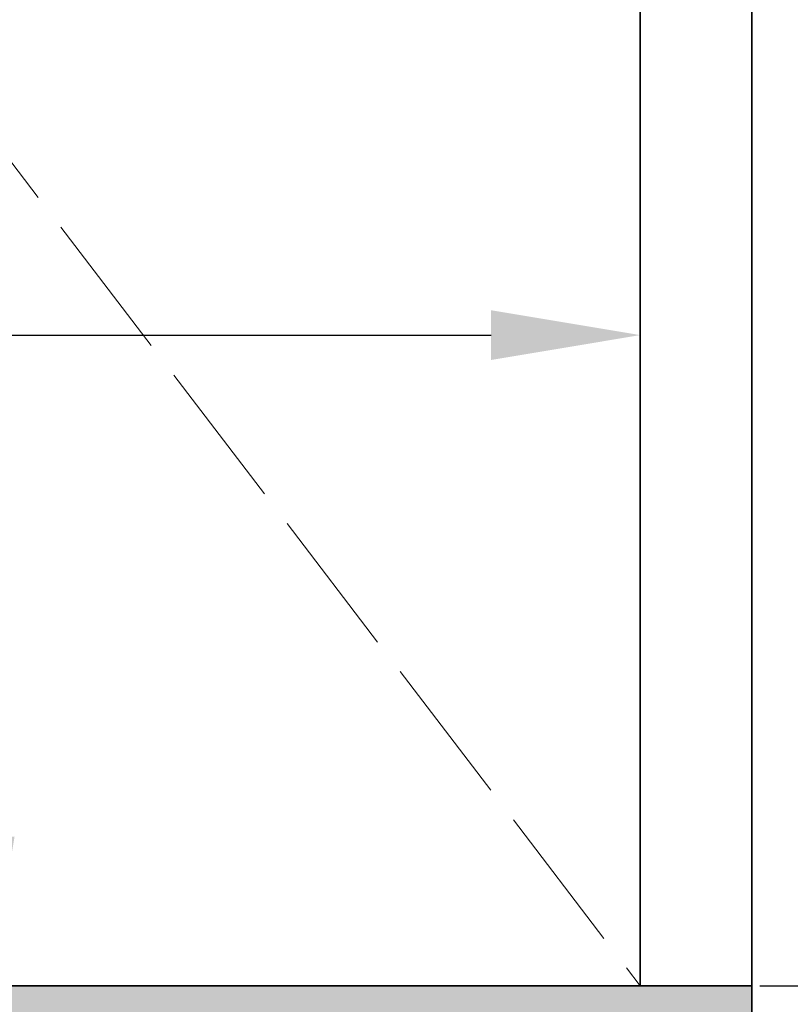
# Model space of a CAD drawing. Units: inches. Extents: x 2083 to 3317, y 1141 to 2115.
# Tile 250 of 256: x 3068 to 3130, y 1485 to 1564. Entities that reach past the tile are written whole.
import ezdxf

# ---------------------------------------------------------------- set-up
doc = ezdxf.new("R2010")
doc.units = ezdxf.units.IN
doc.linetypes.add('ACAD_ISO02W100', pattern=[15, 12, -3])
for name, color, linetype, lineweight in [('A-ANNO-DIMS', 2, 'Continuous', 18), ('A-FLOR-OPEN', 8, 'ACAD_ISO02W100', 13), ('A-WALL', 7, 'Continuous', 35)]:
    doc.layers.add(name, color=color, linetype=linetype, lineweight=lineweight)
doc.layers.add('A-WALL-PATT', color=251, linetype='Continuous', lineweight=13, true_color=0x636466)
doc.styles.get("Standard").update_dxf_attribs({"font": 'arial.ttf'})
doc.dimstyles.new('ISO-25', dxfattribs={"dimtxt": 12, "dimasz": 12, "dimexe": 1.25, "dimexo": 0.625, "dimtad": 1, "dimlunit": 3, "dimtxsty": 'Standard', "dimcen": 2.5, "dimadec": 0, "dimazin": 0, "dimtfac": 1, "dimtmove": 0, "dimatfit": 3, "dimfxl": 1, "dimarcsym": 0})

# ---------------------------------------------------------------- blocks, each defined once
blk = doc.blocks.new('*D8')
at = {"layer": 'A-ANNO-DIMS', "color": 0, "lineweight": -2, "transparency": 16777216}
for p, q in [((3127.585, 1702.761), (3191.318, 1702.761)), ((3190.068, 1690.761), (3190.068, 1498.761)), ((3127.585, 1486.761), (3191.318, 1486.761))]:
    blk.add_line(p, q, dxfattribs=at)
at = {"layer": 'A-ANNO-DIMS', "color": 0, "transparency": 16777216}
for points in [[(3188.068, 1690.761), (3192.068, 1690.761), (3190.068, 1702.761)], [(3188.068, 1498.761), (3192.068, 1498.761), (3190.068, 1486.761)]]:
    blk.add_solid(points, dxfattribs=at)
at = {"layer": 'Defpoints', "color": 0, "transparency": 16777216}
for p in [(3126.96, 1702.761), (3126.96, 1486.761), (3190.068, 1486.761)]:
    blk.add_point(p, dxfattribs=at)
at = {"layer": 'A-ANNO-DIMS', "color": 0, "transparency": 16777216, "insert": (3183.316, 1594.761), "char_height": 12, "attachment_point": 5, "rotation": 90}
blk.add_mtext("18'", dxfattribs=at)
blk = doc.blocks.new('*D9')
at = {"layer": 'A-ANNO-DIMS', "color": 0, "lineweight": -2, "transparency": 16777216}
for p, q in [((3127.585, 1486.761), (3190.403, 1486.761)), ((3189.153, 1474.761), (3189.153, 1275.261)), ((3127.585, 1263.261), (3190.403, 1263.261))]:
    blk.add_line(p, q, dxfattribs=at)
at = {"layer": 'A-ANNO-DIMS', "color": 0, "transparency": 16777216}
for points in [[(3187.153, 1474.761), (3191.153, 1474.761), (3189.153, 1486.761)], [(3187.153, 1275.261), (3191.153, 1275.261), (3189.153, 1263.261)]]:
    blk.add_solid(points, dxfattribs=at)
at = {"layer": 'Defpoints', "color": 0, "transparency": 16777216}
for p in [(3126.96, 1486.761), (3126.96, 1263.261), (3189.153, 1263.261)]:
    blk.add_point(p, dxfattribs=at)
at = {"layer": 'A-ANNO-DIMS', "color": 0, "transparency": 16777216, "insert": (3182.401, 1375.011), "char_height": 12, "attachment_point": 5, "rotation": 90}
blk.add_mtext('18\'-7.5"', dxfattribs=at)
blk = doc.blocks.new('*D35')
at = {"layer": 'A-ANNO-DIMS', "color": 0, "lineweight": -2, "transparency": 16777216}
for p, q in [((3127.585, 2020.761), (3180.56, 2020.761)), ((3179.31, 1275.261), (3179.31, 2008.761)), ((3127.585, 1263.261), (3180.56, 1263.261))]:
    blk.add_line(p, q, dxfattribs=at)
at = {"layer": 'A-ANNO-DIMS', "color": 0, "transparency": 16777216}
for points in [[(3177.31, 2008.761), (3181.31, 2008.761), (3179.31, 2020.761)], [(3177.31, 1275.261), (3181.31, 1275.261), (3179.31, 1263.261)]]:
    blk.add_solid(points, dxfattribs=at)
at = {"layer": 'Defpoints', "color": 0, "transparency": 16777216}
for p in [(3126.96, 2020.761), (3179.31, 2020.761), (3126.96, 1263.261)]:
    blk.add_point(p, dxfattribs=at)
at = {"layer": 'A-ANNO-DIMS', "color": 0, "transparency": 16777216, "insert": (3172.476, 1642.011), "char_height": 12, "attachment_point": 5, "rotation": 90}
blk.add_mtext('63\'-1 1/2"', dxfattribs=at)
blk = doc.blocks.new('*D46')
at = {"layer": 'A-ANNO-DIMS', "color": 0, "lineweight": -2, "transparency": 16777216}
for p, q in [((2952.96, 1487.386), (2952.96, 1540.361)), ((3117.96, 1487.386), (3117.96, 1540.361)), ((2964.96, 1539.111), (3105.96, 1539.111))]:
    blk.add_line(p, q, dxfattribs=at)
at = {"layer": 'A-ANNO-DIMS', "color": 0, "transparency": 16777216}
for points in [[(2964.96, 1541.111), (2964.96, 1537.111), (2952.96, 1539.111)], [(3105.96, 1541.111), (3105.96, 1537.111), (3117.96, 1539.111)]]:
    blk.add_solid(points, dxfattribs=at)
at = {"layer": 'Defpoints', "color": 0, "transparency": 16777216}
for p in [(3117.96, 1539.111), (2952.96, 1486.761), (3117.96, 1486.761)]:
    blk.add_point(p, dxfattribs=at)
at = {"layer": 'A-ANNO-DIMS', "color": 0, "transparency": 16777216, "insert": (3035.46, 1545.867), "char_height": 12, "attachment_point": 5}
blk.add_mtext('13\'-9"', dxfattribs=at)
blk = doc.blocks.new('*D65')
at = {"layer": 'A-ANNO-DIMS', "color": 0, "lineweight": -2, "transparency": 16777216}
for p, q in [((3117.335, 1702.761), (3064.36, 1702.761)), ((3065.61, 1498.761), (3065.61, 1690.761)), ((3117.335, 1486.761), (3064.36, 1486.761))]:
    blk.add_line(p, q, dxfattribs=at)
at = {"layer": 'A-ANNO-DIMS', "color": 0, "transparency": 16777216}
for points in [[(3063.61, 1690.761), (3067.61, 1690.761), (3065.61, 1702.761)], [(3063.61, 1498.761), (3067.61, 1498.761), (3065.61, 1486.761)]]:
    blk.add_solid(points, dxfattribs=at)
at = {"layer": 'Defpoints', "color": 0, "transparency": 16777216}
for p in [(3065.61, 1702.761), (3117.96, 1702.761), (3117.96, 1486.761)]:
    blk.add_point(p, dxfattribs=at)
at = {"layer": 'A-ANNO-DIMS', "color": 0, "transparency": 16777216, "insert": (3058.858, 1594.761), "char_height": 12, "attachment_point": 5, "rotation": 90}
blk.add_mtext('18\'-0"', dxfattribs=at)

msp = doc.modelspace()

# ---------------------------------------------------------------- hatches: boundary and pattern name
at = {"layer": 'A-WALL-PATT'}
h = msp.add_hatch(color=256, dxfattribs=at)
h.dxf.hatch_style = 1
h.paths.add_polyline_path([(3126.96, 2020.761), (2748.96, 2020.761), (2604.96, 2020.761), (2226.96, 2020.761), (2226.96, 1702.761), (2466.96, 1702.761), (2466.96, 1582.761), (2418.96, 1582.761), (2418.96, 1477.761), (2226.96, 1477.761), (2226.96, 1263.261), (2544.96, 1263.261), (2544.96, 1411.761), (2604.96, 1411.761), (2685.96, 1411.761), (2685.96, 1420.761), (2604.96, 1420.761), (2604.96, 1573.761), (2604.96, 1702.761), (2604.96, 2011.761), (2748.96, 2011.761), (2748.96, 1702.761), (2862.96, 1702.761), (2862.96, 1621.761), (2871.96, 1621.761), (2871.96, 1702.761), (2883.96, 1702.761), (2883.96, 1706.939, -0.026459), (2883.96, 1711.761), (2757.96, 1711.761), (2757.96, 1807.761), (2787.96, 1807.761), (2787.96, 1812.261), (2757.96, 1812.261), (2757.96, 2011.761), (2877.96, 2011.761), (2877.96, 1812.261), (2847.96, 1812.261), (2847.96, 1807.761), (2889.836, 1807.761), (2889.836, 1812.261), (2882.46, 1812.261), (2882.46, 2011.761), (3117.96, 2011.761), (3117.96, 1812.261), (2937.836, 1812.261), (2937.836, 1807.761), (2995.71, 1807.761), (2995.71, 1796.118), (3000.21, 1796.118), (3000.21, 1807.761), (3117.96, 1807.761), (3117.96, 1711.761), (3000.21, 1711.761), (3000.21, 1760.118), (2998.573, 1760.118, -0.020711), (2995.71, 1760.118), (2995.71, 1711.761), (2931.96, 1711.761), (2931.96, 1702.761), (3126.96, 1702.761)])
h.paths.add_polyline_path([(2471.46, 2011.761), (2471.46, 1810.011), (2462.717, 1810.011), (2462.717, 1805.511), (2505.96, 1805.511), (2505.96, 1810.011), (2475.96, 1810.011), (2475.96, 2011.761), (2595.96, 2011.761), (2595.96, 1810.011), (2565.96, 1810.011), (2565.96, 1805.511), (2595.96, 1805.511), (2595.96, 1711.761), (2235.96, 1711.761), (2235.96, 1805.511), (2353.71, 1805.511), (2353.71, 1796.054), (2358.21, 1796.054), (2358.21, 1805.511), (2414.717, 1805.511), (2414.717, 1810.011), (2235.96, 1810.011), (2235.96, 2011.761)], flags=16)
h.paths.add_polyline_path([(2270.205, 1994.61), (2270.205, 1970.61), (2246.205, 1970.61), (2246.205, 1994.61)], flags=0)
edge = h.paths.add_edge_path(flags=0)
edge.add_ellipse((2332.027, 1899.798), major_axis=(-3.043, 3.043), ratio=0.168252, start_angle=-161.33217, end_angle=-156.30711, ccw=False)
edge.add_ellipse((2333.082, 1898.744), major_axis=(-1.055, 1.055), ratio=0.453532, start_angle=-123.37102, end_angle=-94.15911)
edge = h.paths.add_edge_path(flags=0)
edge.add_ellipse((2332.027, 1968.876), major_axis=(3.043, 3.043), ratio=0.168252, start_angle=18.66783, end_angle=23.69289)
edge.add_spline(control_points=[(2332.926, 1970.691), (2332.227, 1970.336), (2330.894, 1969.659), (2328.413, 1970.932), (2327.204, 1967.749), (2324.71, 1969.956), (2322.533, 1967.012), (2320.013, 1971.296), (2317.68, 1968.158), (2316.041, 1967.102), (2315.427, 1966.81)], knot_values=[0, 0, 0, 0, 2.267059, 4.324559, 6.685584, 8.878641, 11.121502, 14.300359, 17.755284, 19.732645, 19.732645, 19.732645, 19.732645], degree=3, periodic=0)
edge.add_ellipse((2332.027, 1968.876), major_axis=(3.043, 3.043), ratio=0.168252, start_angle=18.66783, end_angle=23.69289, ccw=False)
edge.add_ellipse((2333.082, 1969.931), major_axis=(1.055, 1.055), ratio=0.453532, start_angle=56.62898, end_angle=85.84089, ccw=False)
edge = h.paths.add_edge_path(flags=0)
edge.add_spline(control_points=[(2296.428, 1967.988), (2293.628, 1965.336), (2287.704, 1959.727), (2299.744, 1949.996), (2294.533, 1935.669), (2290.573, 1920.604), (2293.394, 1909.974), (2296.185, 1904.967)], knot_values=[0.099185, 0.099185, 0.099185, 0.099185, 0.345301, 0.619822, 0.982653, 1.386093, 1.810555, 1.810555, 1.810555, 1.810555], degree=3, periodic=0)
edge.add_spline(control_points=[(2296.185, 1904.967), (2297.384, 1902.619), (2298.001, 1901.949), (2298.553, 1901.468)], knot_values=[0.006246, 0.006246, 0.006246, 0.006246, 0.055476, 0.055476, 0.055476, 0.055476], degree=3, periodic=0)
edge.add_spline(control_points=[(2298.553, 1901.468), (2297.259, 1900.923), (2295.225, 1900.232), (2293.06, 1900.614), (2292.101, 1900.788), (2292.09, 1900.791)], knot_values=[0.312835, 0.312835, 0.312835, 0.312835, 0.40178, 0.474987, 0.475903, 0.475903, 0.475903, 0.475903], degree=3, periodic=0)
edge.add_arc((2292.794, 1904.664), 3.937, 215.4209, 259.69818, ccw=False)
edge.add_spline(control_points=[(2289.585, 1902.382), (2289.477, 1902.535), (2289.368, 1902.688), (2289.261, 1902.841)], knot_values=[0.102872, 0.102872, 0.102872, 0.102872, 0.116896, 0.116896, 0.116896, 0.116896], degree=3, periodic=0)
edge.add_spline(control_points=[(2289.261, 1902.841), (2288.687, 1902.55), (2287.64, 1902.02), (2285.881, 1901.874), (2283.853, 1901.504), (2281.72, 1899.711), (2278.467, 1899.493), (2276.157, 1901.883), (2272.259, 1899.804), (2267.778, 1901.843), (2262.244, 1900.184), (2257.415, 1901.782), (2254.318, 1900.726), (2253.178, 1900.337)], knot_values=[0, 0, 0, 0, 1.907977, 3.477176, 5.261074, 7.972851, 11.680248, 13.717921, 16.939592, 22.789562, 27.502503, 33.595215, 37.145618, 37.145618, 37.145618, 37.145618], degree=3, periodic=0)
edge.add_line((2253.178, 1900.337), (2250.244, 1902.841))
edge.add_line((2250.244, 1902.841), (2250.244, 1965.833))
edge.add_line((2250.244, 1965.833), (2253.178, 1968.337))
edge.add_spline(control_points=[(2253.178, 1968.337), (2254.318, 1967.948), (2257.415, 1966.892), (2262.244, 1968.49), (2267.778, 1966.831), (2271.527, 1968.537), (2273.876, 1967.828), (2274.207, 1967.728)], knot_values=[0, 0, 0, 0, 0.09018, 0.244935, 0.364644, 0.513233, 0.537855, 0.537855, 0.537855, 0.537855], degree=3, periodic=0)
edge.add_arc((2274.353, 1963.793), 3.937, 72.05113, 92.12795, ccw=False)
edge.add_arc((2281.297, 1985.23), 18.596, 252.05113, 288.56572)
edge.add_arc((2292.317, 1956.029), 12.646, 71.02679, 113.77822, ccw=False)
edge = h.paths.add_edge_path(flags=0)
edge.add_spline(control_points=[(2274.899, 1951.856), (2275.066, 1951.617), (2275.233, 1951.377), (2275.398, 1951.136)], knot_values=[1.409916, 1.409916, 1.409916, 1.409916, 1.43159, 1.43159, 1.43159, 1.43159], degree=3, periodic=0)
edge.add_spline(control_points=[(2275.398, 1951.136), (2275.792, 1950.562), (2276.179, 1949.984), (2276.546, 1949.397)], knot_values=[1.358238, 1.358238, 1.358238, 1.358238, 1.409916, 1.409916, 1.409916, 1.409916], degree=3, periodic=0)
edge.add_line((2276.546, 1949.397), (2277.437, 1947.862))
edge.add_spline(control_points=[(2277.437, 1947.862), (2276.304, 1945.673), (2274.64, 1942.427), (2274.632, 1938.094), (2272.799, 1930.852), (2274.356, 1943.897), (2275.948, 1947.923), (2276.546, 1949.397)], knot_values=[0.005632, 0.005632, 0.005632, 0.005632, 0.186014, 0.266002, 0.357087, 0.59639, 0.739732, 0.739732, 0.739732, 0.739732], degree=3, periodic=0)
edge.add_spline(control_points=[(2276.546, 1949.397), (2276.179, 1949.984), (2275.792, 1950.562), (2275.398, 1951.136)], knot_values=[1.358238, 1.358238, 1.358238, 1.358238, 1.409916, 1.409916, 1.409916, 1.409916], degree=3, periodic=0)
edge.add_spline(control_points=[(2275.398, 1951.136), (2274.943, 1950.08), (2274.208, 1948.025), (2273.935, 1944.851), (2272.469, 1937.627), (2273.466, 1945.696), (2274.701, 1951.059), (2274.899, 1951.856)], knot_values=[0.104364, 0.104364, 0.104364, 0.104364, 0.189636, 0.269624, 0.36071, 0.600013, 0.644622, 0.644622, 0.644622, 0.644622], degree=3, periodic=0)
h.paths.add_polyline_path([(2269.168, 1963.128, -0.357527), (2268.171, 1960.976, -0.092561), (2268.171, 1939.436, -0.357527), (2269.168, 1937.285, -0.357527), (2267.016, 1938.282, -0.164785), (2254.686, 1938.282, -0.357527), (2252.534, 1937.285, -0.357527), (2253.531, 1939.436, -0.092561), (2253.531, 1960.976, -0.357527), (2252.534, 1963.128, -0.357527), (2254.686, 1962.131, -0.164785), (2267.016, 1962.131, -0.357527)], flags=0)
h.paths.add_polyline_path([(2248.874, 1967.802), (2248.874, 1957.028), (2249.458, 1957.028), (2249.458, 1911.647), (2248.874, 1911.647), (2248.874, 1900.873), (2246.512, 1900.873, 0.197327), (2244.15, 1902.457), (2244.15, 1966.218, 0.197327), (2246.512, 1967.802)], flags=0)
h.paths.add_polyline_path([(2269.168, 1931.389, -0.357527), (2268.171, 1929.238, -0.092561), (2268.171, 1907.698, -0.357527), (2269.168, 1905.547, -0.357527), (2267.016, 1906.544, -0.164785), (2254.686, 1906.544, -0.357527), (2252.534, 1905.547, -0.357527), (2253.531, 1907.698, -0.092561), (2253.531, 1929.238, -0.357527), (2252.534, 1931.389, -0.357527), (2254.686, 1930.392, -0.164785), (2267.016, 1930.392, -0.357527)], flags=0)
edge = h.paths.add_edge_path(flags=0)
edge.add_spline(control_points=[(2276.197, 1906.724), (2276.168, 1909.029), (2276.114, 1913.372), (2270.598, 1924.925), (2273.905, 1919.013), (2275.922, 1916.262), (2275.475, 1912.402), (2277.258, 1910.381), (2276.696, 1908.225), (2276.646, 1906.813), (2276.618, 1906.008)], knot_values=[0, 0, 0, 0, 8.61026, 16.221274, 18.843057, 23.804898, 27.440828, 29.356102, 31.203478, 33.650687, 33.650687, 33.650687, 33.650687], degree=3, periodic=0)
edge.add_spline(control_points=[(2276.618, 1906.008), (2276.623, 1905.624), (2276.498, 1904.629), (2275.442, 1903.855), (2274.937, 1903.08), (2274.859, 1902.841)], knot_values=[0.156488, 0.156488, 0.156488, 0.156488, 0.184398, 0.231376, 0.250598, 0.250598, 0.250598, 0.250598], degree=3, periodic=0)
edge.add_line((2274.859, 1902.841), (2276.506, 1902.841))
edge.add_spline(control_points=[(2276.506, 1902.841), (2276.788, 1903.085), (2277.665, 1904.125), (2278.25, 1904.341), (2277.654, 1908.527), (2278.156, 1906.228), (2278.1, 1905.286), (2278.847, 1904.069), (2277.857, 1903.415), (2277.874, 1902.991), (2277.904, 1902.841)], knot_values=[0.059574, 0.059574, 0.059574, 0.059574, 0.080753, 0.103741, 0.16972, 0.176036, 0.207137, 0.240474, 0.262341, 0.27366, 0.27366, 0.27366, 0.27366], degree=3, periodic=0)
edge.add_line((2277.904, 1902.841), (2280.03, 1902.841))
edge.add_spline(control_points=[(2280.03, 1902.841), (2279.888, 1903.088), (2279.499, 1903.982), (2280.152, 1905.939), (2278.104, 1909.658), (2279.762, 1907.185), (2280.328, 1904.875), (2280.485, 1903.49), (2281.463, 1903.249), (2281.758, 1902.936), (2281.834, 1902.841)], knot_values=[0.013856, 0.013856, 0.013856, 0.013856, 0.034874, 0.088867, 0.107879, 0.126738, 0.158714, 0.193757, 0.217487, 0.226722, 0.226722, 0.226722, 0.226722], degree=3, periodic=0)
edge.add_spline(control_points=[(2281.834, 1902.841), (2281.788, 1902.827), (2281.647, 1902.783), (2281.396, 1902.859), (2281.088, 1902.985), (2280.721, 1903.061), (2280.333, 1903.026), (2280.125, 1902.899), (2280.03, 1902.841)], knot_values=[0, 0, 0, 0, 0.14413, 0.435517, 0.749276, 1.153046, 1.548371, 1.878348, 1.878348, 1.878348, 1.878348], degree=3, periodic=0)
edge.add_line((2280.03, 1902.841), (2277.904, 1902.841))
edge.add_spline(control_points=[(2277.904, 1902.841), (2277.893, 1902.796), (2277.865, 1902.68), (2277.607, 1902.687), (2277.274, 1902.801), (2276.838, 1902.62), (2276.584, 1902.789), (2276.506, 1902.841)], knot_values=[0, 0, 0, 0, 0.127189, 0.326199, 0.628009, 1.24357, 1.515331, 1.515331, 1.515331, 1.515331], degree=3, periodic=0)
edge.add_line((2276.506, 1902.841), (2274.859, 1902.841))
edge.add_spline(control_points=[(2274.859, 1902.841), (2274.814, 1902.899), (2274.725, 1903.013), (2274.493, 1903.119), (2274.244, 1902.961), (2273.937, 1903.185), (2273.614, 1902.983), (2273.408, 1902.883), (2273.322, 1902.841)], knot_values=[0, 0, 0, 0, 0.21843, 0.436957, 0.687977, 0.990379, 1.398396, 1.69185, 1.69185, 1.69185, 1.69185], degree=3, periodic=0)
edge.add_spline(control_points=[(2273.322, 1902.841), (2273.617, 1903.446), (2274.274, 1904.538), (2276.027, 1904.574), (2276.207, 1906.584), (2276.197, 1906.724)], knot_values=[0.012227, 0.012227, 0.012227, 0.012227, 0.059472, 0.106218, 0.134458, 0.134458, 0.134458, 0.134458], degree=3, periodic=0)
h.paths.add_polyline_path([(2270.776, 1897.79), (2270.776, 1873.79), (2246.776, 1873.79), (2246.776, 1897.79)], flags=0)
h.paths.add_polyline_path([(2353.71, 1760.005), (2353.71, 1760.054), (2358.21, 1760.054, -0.033729)], flags=0)
h.paths.add_polyline_path([(2321.819, 1737.529), (2341.995, 1737.529, -0.414214), (2343.203, 1736.321), (2343.203, 1721.021, -0.414214), (2341.995, 1719.813), (2321.819, 1719.813, -0.414214), (2320.611, 1721.021), (2320.611, 1736.321, -0.414214)], flags=0)
h.paths.add_polyline_path([(2324.235, 1736.321), (2339.579, 1736.321, -0.414214), (2341.995, 1733.905), (2341.995, 1725.45, -0.414214), (2339.579, 1723.034), (2333.681, 1723.034), (2333.845, 1722.045, -0.870646), (2335.425, 1721.826, -0.767327), (2333.923, 1721.423), (2331.291, 1721.423, -0.767327), (2329.788, 1721.826, -0.870646), (2331.368, 1722.045), (2331.533, 1723.034), (2324.235, 1723.034, -0.414214), (2321.819, 1725.45), (2321.819, 1733.905, -0.414214)], flags=0)
h.paths.add_polyline_path([(2570.484, 1928.615), (2589.684, 1928.615), (2590.169, 1928.615), (2590.169, 1904.993), (2570.484, 1904.993)], flags=0)
h.paths.add_polyline_path([(2574.447, 1927.264, -1), (2572.829, 1927.264, -1)], flags=0)
h.paths.add_polyline_path([(2573.09, 1926.941), (2573.925, 1927.776), (2574.148, 1927.553), (2573.313, 1926.718)], flags=0)
h.paths.add_polyline_path([(2578.779, 1919.73, -1), (2571.592, 1919.73, -1)], flags=0)
h.paths.add_polyline_path([(2578.385, 1919.73, -1), (2571.985, 1919.73, -1)], flags=0)
h.paths.add_polyline_path([(2331.596, 1729.476, -1), (2333.618, 1729.476, -1)], flags=0)
h.paths.add_polyline_path([(2578.034, 1927.264, -1), (2576.416, 1927.264, -1)], flags=0)
h.paths.add_polyline_path([(2576.689, 1927.531), (2576.912, 1927.754), (2577.747, 1926.919), (2577.524, 1926.696)], flags=0)
h.paths.add_polyline_path([(2578.139, 1909.86, -1), (2572.232, 1909.86, -1)], flags=0)
h.paths.add_polyline_path([(2577.745, 1909.86, -1), (2572.625, 1909.86, -1)], flags=0)
h.paths.add_polyline_path([(2583.798, 1927.264, -1), (2582.179, 1927.264, -1)], flags=0)
h.paths.add_polyline_path([(2582.719, 1927.754), (2583.554, 1926.919), (2583.331, 1926.696), (2582.496, 1927.531)], flags=0)
h.paths.add_polyline_path([(2582.496, 1927.531), (2582.719, 1927.754), (2583.554, 1926.919), (2583.331, 1926.696)], flags=0)
h.paths.add_polyline_path([(2587.739, 1920.53, -1), (2581.832, 1920.53, -1)], flags=0)
h.paths.add_polyline_path([(2587.345, 1920.53, -1), (2582.225, 1920.53, -1)], flags=0)
h.paths.add_polyline_path([(2587.385, 1927.264, -1), (2585.766, 1927.264, -1)], flags=0)
h.paths.add_polyline_path([(2586.082, 1926.98), (2586.917, 1927.815), (2587.14, 1927.593), (2586.305, 1926.758)], flags=0)
h.paths.add_polyline_path([(2588.379, 1910.66, -1), (2581.192, 1910.66, -1)], flags=0)
h.paths.add_polyline_path([(2587.985, 1910.66, -1), (2581.585, 1910.66, -1)], flags=0)
h.paths.add_polyline_path([(2417.168, 1729.478), (2437.344, 1729.478, -0.414214), (2438.552, 1728.27), (2438.552, 1712.969, -0.414214), (2437.344, 1711.761), (2417.168, 1711.761, -0.414214), (2415.96, 1712.969), (2415.96, 1728.27, -0.414214)], flags=0)
h.paths.add_polyline_path([(2419.584, 1728.27), (2434.928, 1728.27, -0.414214), (2437.344, 1725.854), (2437.344, 1717.398, -0.414214), (2434.928, 1714.983), (2429.029, 1714.983), (2429.194, 1713.994, -0.870646), (2430.774, 1713.775, -0.767327), (2429.271, 1713.372), (2426.64, 1713.372, -0.767327), (2425.137, 1713.775, -0.870646), (2426.717, 1713.994), (2426.882, 1714.983), (2419.584, 1714.983, -0.414214), (2417.168, 1717.398), (2417.168, 1725.854, -0.414214)], flags=0)
h.paths.add_polyline_path([(2419.584, 1728.27), (2434.928, 1728.27, -0.414214), (2437.344, 1725.854), (2437.344, 1717.398, -0.414214), (2434.928, 1714.983), (2429.029, 1714.983), (2428.358, 1719.009), (2427.553, 1719.009), (2426.882, 1714.983), (2419.584, 1714.983, -0.414214), (2417.168, 1717.398), (2417.168, 1725.854, -0.414214)], flags=0)
h.paths.add_polyline_path([(2426.944, 1721.425, -1), (2428.967, 1721.425, -1)], flags=0)
h.paths.add_polyline_path([(2475.96, 1702.761), (2595.96, 1702.761), (2595.96, 1582.761), (2475.96, 1582.761)], flags=16)
h.paths.add_polyline_path([(2427.96, 1573.761), (2595.96, 1573.761), (2595.96, 1468.761), (2595.96, 1420.761), (2384.46, 1420.761), (2384.46, 1468.761), (2427.96, 1468.761)], flags=16)
h.paths.add_polyline_path([(2379.96, 1468.761), (2379.96, 1420.761), (2235.96, 1420.761), (2235.96, 1468.761)], flags=16)
h.paths.add_polyline_path([(2317.816, 1466.696), (2337.992, 1466.696, -0.414214), (2339.2, 1465.488), (2339.2, 1450.187, -0.414214), (2337.992, 1448.979), (2317.816, 1448.979, -0.414214), (2316.608, 1450.187), (2316.608, 1465.488, -0.414214)], flags=0)
h.paths.add_polyline_path([(2320.232, 1465.488), (2335.576, 1465.488, -0.414214), (2337.992, 1463.072), (2337.992, 1454.616, -0.414214), (2335.576, 1452.2), (2329.677, 1452.2), (2329.842, 1451.212, -0.870646), (2331.422, 1450.992, -0.767327), (2329.92, 1450.59), (2327.288, 1450.59, -0.767327), (2325.785, 1450.992, -0.870646), (2327.365, 1451.212), (2327.53, 1452.2), (2320.232, 1452.2, -0.414214), (2317.816, 1454.616), (2317.816, 1463.072, -0.414214)], flags=0)
h.paths.add_polyline_path([(2320.232, 1465.488), (2335.576, 1465.488, -0.414214), (2337.992, 1463.072), (2337.992, 1454.616, -0.414214), (2335.576, 1452.2), (2329.677, 1452.2), (2329.006, 1456.227), (2328.201, 1456.227), (2327.53, 1452.2), (2320.232, 1452.2, -0.414214), (2317.816, 1454.616), (2317.816, 1463.072, -0.414214)], flags=0)
h.paths.add_polyline_path([(2327.593, 1458.643, -1), (2329.615, 1458.643, -1)], flags=0)
h.paths.add_polyline_path([(2244.412, 1433.34), (2241.921, 1433.34, -0.414214), (2240.018, 1435.244), (2240.018, 1440.953, -0.414211), (2241.921, 1442.856), (2244.412, 1442.856, -1.976472)], flags=0)
h.paths.add_polyline_path([(2245.357, 1434.398, -0.414214), (2245.357, 1441.799, -2.144098)], flags=0)
h.paths.add_polyline_path([(2535.96, 1416.261), (2535.96, 1272.261), (2235.96, 1272.261), (2235.96, 1416.261)], flags=16)
h.paths.add_polyline_path([(2260.12, 1384.293), (2260.12, 1362.039), (2237.865, 1362.039), (2237.865, 1384.293)], flags=0)
edge = h.paths.add_edge_path(flags=0)
edge.add_line((2318.252, 1362.093), (2318.146, 1362.001))
edge.add_ellipse((2317.445, 1360.431), major_axis=(2.822, 2.822), ratio=0.168252, start_angle=18.66783, end_angle=20.94813, ccw=False)
edge.add_ellipse((2318.423, 1361.409), major_axis=(0.978, 0.978), ratio=0.453532, start_angle=56.62898, end_angle=70.2262, ccw=False)
edge = h.paths.add_edge_path(flags=0)
edge.add_line((2319.107, 1295.571), (2319.015, 1295.677))
edge.add_ellipse((2317.445, 1296.378), major_axis=(-2.822, 2.822), ratio=0.168252, start_angle=-161.33217, end_angle=-159.05187, ccw=False)
edge.add_ellipse((2318.423, 1295.4), major_axis=(-0.978, 0.978), ratio=0.453532, start_angle=-123.37102, end_angle=-109.7738)
edge = h.paths.add_edge_path(flags=0)
edge.add_spline(control_points=[(2284.21, 1301.17), (2284.581, 1300.445), (2284.891, 1299.892), (2285.16, 1299.461)], knot_values=[0.039066, 0.039066, 0.039066, 0.039066, 0.055476, 0.055476, 0.055476, 0.055476], degree=3, periodic=0)
edge.add_line((2285.16, 1299.461), (2284.21, 1301.17))
edge = h.paths.add_edge_path(flags=0)
edge.add_line((2280.412, 1297.298), (2283.37, 1297.036))
edge.add_line((2283.37, 1297.036), (2286.406, 1297.926))
edge.add_spline(control_points=[(2286.406, 1297.926), (2285.305, 1297.463), (2284.345, 1297.129), (2283.37, 1297.036)], knot_values=[0.394369, 0.394369, 0.394369, 0.394369, 0.475903, 0.475903, 0.475903, 0.475903], degree=3, periodic=0)
edge.add_spline(control_points=[(2283.37, 1297.036), (2283.281, 1297.028), (2282.316, 1296.957), (2281.313, 1297.134), (2280.423, 1297.296), (2280.412, 1297.298)], knot_values=[0.312835, 0.312835, 0.312835, 0.312835, 0.320246, 0.393453, 0.394369, 0.394369, 0.394369, 0.394369], degree=3, periodic=0)
edge = h.paths.add_edge_path(flags=0)
edge.add_line((2284.436, 1359.607), (2280.446, 1355.328))
edge.add_line((2280.446, 1355.328), (2279.58, 1351.018))
edge.add_line((2279.58, 1351.018), (2282.413, 1346.58))
edge.add_spline(control_points=[(2282.413, 1346.58), (2283.153, 1345.589), (2284.253, 1344.029), (2284.801, 1342.387), (2284.935, 1341.806)], knot_values=[1.240098, 1.240098, 1.240098, 1.240098, 1.332892, 1.382712, 1.382712, 1.382712, 1.382712], degree=3, periodic=0)
edge.add_spline(control_points=[(2284.935, 1341.806), (2285.319, 1340.141), (2285.233, 1338.409), (2284.91, 1336.654)], knot_values=[1.097484, 1.097484, 1.097484, 1.097484, 1.240098, 1.240098, 1.240098, 1.240098], degree=3, periodic=0)
edge.add_spline(control_points=[(2284.91, 1336.654), (2284.587, 1334.899), (2284.027, 1333.12), (2283.463, 1331.361)], knot_values=[0.95487, 0.95487, 0.95487, 0.95487, 1.097484, 1.097484, 1.097484, 1.097484], degree=3, periodic=0)
edge.add_line((2283.463, 1331.361), (2281.89, 1326.153))
edge.add_line((2281.89, 1326.153), (2280.756, 1321.056))
edge.add_line((2280.756, 1321.056), (2280.299, 1316.002))
edge.add_line((2280.299, 1316.002), (2280.716, 1310.95))
edge.add_line((2280.716, 1310.95), (2282.028, 1305.972))
edge.add_line((2282.028, 1305.972), (2284.21, 1301.17))
edge.add_spline(control_points=[(2284.21, 1301.17), (2283.341, 1302.73), (2282.612, 1304.336), (2282.028, 1305.972)], knot_values=[0.099185, 0.099185, 0.099185, 0.099185, 0.241799, 0.241799, 0.241799, 0.241799], degree=3, periodic=0)
edge.add_spline(control_points=[(2282.028, 1305.972), (2281.444, 1307.608), (2281.005, 1309.273), (2280.716, 1310.95)], knot_values=[0.241799, 0.241799, 0.241799, 0.241799, 0.384413, 0.384413, 0.384413, 0.384413], degree=3, periodic=0)
edge.add_spline(control_points=[(2280.716, 1310.95), (2280.433, 1312.588), (2280.289, 1314.277), (2280.299, 1315.962), (2280.299, 1316.002)], knot_values=[0.384413, 0.384413, 0.384413, 0.384413, 0.523647, 0.527028, 0.527028, 0.527028, 0.527028], degree=3, periodic=0)
edge.add_spline(control_points=[(2280.299, 1316.002), (2280.312, 1317.687), (2280.478, 1319.368), (2280.756, 1321.056)], knot_values=[0.527028, 0.527028, 0.527028, 0.527028, 0.669642, 0.669642, 0.669642, 0.669642], degree=3, periodic=0)
edge.add_spline(control_points=[(2280.756, 1321.056), (2281.035, 1322.744), (2281.426, 1324.44), (2281.89, 1326.153)], knot_values=[0.669642, 0.669642, 0.669642, 0.669642, 0.812256, 0.812256, 0.812256, 0.812256], degree=3, periodic=0)
edge.add_spline(control_points=[(2281.89, 1326.153), (2282.264, 1327.533), (2282.788, 1329.262), (2283.353, 1331.018), (2283.463, 1331.361)], knot_values=[0.812256, 0.812256, 0.812256, 0.812256, 0.927087, 0.95487, 0.95487, 0.95487, 0.95487], degree=3, periodic=0)
edge.add_line((2283.463, 1331.361), (2284.91, 1336.654))
edge.add_line((2284.91, 1336.654), (2284.935, 1341.806))
edge.add_line((2284.935, 1341.806), (2282.413, 1346.58))
edge.add_spline(control_points=[(2282.413, 1346.58), (2281.275, 1348.104), (2280.078, 1349.57), (2279.58, 1351.018)], knot_values=[1.382712, 1.382712, 1.382712, 1.382712, 1.525326, 1.525326, 1.525326, 1.525326], degree=3, periodic=0)
edge.add_spline(control_points=[(2279.58, 1351.018), (2279.443, 1351.415), (2279.136, 1352.857), (2279.735, 1354.29), (2280.446, 1355.328)], knot_values=[1.525326, 1.525326, 1.525326, 1.525326, 1.564439, 1.667941, 1.667941, 1.667941, 1.667941], degree=3, periodic=0)
edge.add_spline(control_points=[(2280.446, 1355.328), (2281.426, 1356.758), (2282.931, 1358.183), (2284.436, 1359.607)], knot_values=[1.667941, 1.667941, 1.667941, 1.667941, 1.810555, 1.810555, 1.810555, 1.810555], degree=3, periodic=0)
edge.add_arc((2280.623, 1348.518), 11.726, 71.02679, 113.77822)
edge.add_arc((2270.405, 1375.595), 17.244, 252.05113, 288.56572, ccw=False)
edge.add_arc((2263.966, 1355.718), 3.651, 72.05113, 92.12795)
edge.add_arc((2263.966, 1355.718), 3.651, 92.12795, 177.98513)
edge.add_spline(control_points=[(2260.318, 1355.846), (2260.26, 1354.221), (2260.551, 1350.187), (2262.999, 1346.766), (2264.473, 1344.649)], knot_values=[1.43159, 1.43159, 1.43159, 1.43159, 1.564144, 1.770695, 1.770695, 1.770695, 1.770695], degree=3, periodic=0)
edge.add_line((2264.473, 1344.649), (2264.936, 1343.983))
edge.add_spline(control_points=[(2263.801, 1340.248), (2263.843, 1340.514), (2264.067, 1341.756), (2264.513, 1343.002), (2264.935, 1343.981)], knot_values=[0.53657, 0.53657, 0.53657, 0.53657, 0.559349, 0.644622, 0.644622, 0.644622, 0.644622], degree=3, periodic=0)
edge.add_spline(control_points=[(2264.935, 1343.981), (2265.118, 1343.715), (2265.299, 1343.448), (2265.477, 1343.179)], knot_values=[1.384077, 1.384077, 1.384077, 1.384077, 1.409916, 1.409916, 1.409916, 1.409916], degree=3, periodic=0)
edge.add_spline(control_points=[(2265.477, 1343.179), (2265.655, 1342.911), (2265.829, 1342.641), (2265.999, 1342.369)], knot_values=[1.358238, 1.358238, 1.358238, 1.358238, 1.384077, 1.384077, 1.384077, 1.384077], degree=3, periodic=0)
edge.add_line((2265.999, 1342.369), (2266.826, 1340.946))
edge.add_spline(control_points=[(2266.826, 1340.946), (2268.894, 1337.09), (2271.398, 1325.843), (2270.516, 1310.569), (2275.919, 1301.861), (2277.79, 1299.199)], knot_values=[0.116896, 0.116896, 0.116896, 0.116896, 0.472987, 1.050969, 1.313793, 1.313793, 1.313793, 1.313793], degree=3, periodic=0)
edge.add_spline(control_points=[(2277.79, 1299.199), (2277.839, 1299.128), (2277.889, 1299.057), (2277.94, 1298.987)], knot_values=[0.109884, 0.109884, 0.109884, 0.109884, 0.116896, 0.116896, 0.116896, 0.116896], degree=3, periodic=0)
edge.add_line((2277.94, 1298.987), (2277.789, 1299.199))
edge.add_spline(control_points=[(2277.789, 1299.199), (2277.257, 1298.929), (2276.286, 1298.438), (2275.039, 1298.334), (2274.383, 1298.239), (2274.215, 1298.209)], knot_values=[33.12187, 33.12187, 33.12187, 33.12187, 35.029056, 36.598255, 37.144827, 37.144827, 37.144827, 37.144827], degree=3, periodic=0)
edge.add_line((2274.215, 1298.209), (2273.073, 1297.893))
edge.add_spline(control_points=[(2273.073, 1297.893), (2272.323, 1297.58), (2271.039, 1296.511), (2269.248, 1296.226), (2268.423, 1296.375)], knot_values=[26.532584, 26.532584, 26.532584, 26.532584, 29.198919, 31.839101, 31.839101, 31.839101, 31.839101], degree=3, periodic=0)
edge.add_line((2268.423, 1296.375), (2263.879, 1297.458))
edge.add_spline(control_points=[(2263.879, 1297.458), (2263.556, 1297.359), (2261.86, 1296.839), (2260.239, 1297.282), (2258.933, 1297.516)], knot_values=[15.919551, 15.919551, 15.919551, 15.919551, 16.939592, 21.226067, 21.226067, 21.226067, 21.226067], degree=3, periodic=0)
edge.add_line((2258.933, 1297.516), (2254.055, 1297.329))
edge.add_spline(control_points=[(2254.055, 1297.329), (2253.756, 1297.296), (2252.114, 1297.165), (2250.462, 1297.544), (2249.13, 1297.668)], knot_values=[5.306517, 5.306517, 5.306517, 5.306517, 6.276435, 10.613034, 10.613034, 10.613034, 10.613034], degree=3, periodic=0)
edge.add_line((2249.13, 1297.668), (2244.332, 1296.878))
edge.add_line((2244.332, 1296.878), (2241.611, 1299.199))
edge.add_line((2241.611, 1299.199), (2241.611, 1357.609))
edge.add_line((2241.611, 1357.609), (2244.332, 1359.931))
edge.add_line((2244.332, 1359.931), (2252.729, 1359.543))
edge.add_spline(control_points=[(2252.729, 1359.543), (2252.871, 1359.546), (2253.306, 1359.548), (2253.74, 1359.514), (2254.032, 1359.482)], knot_values=[0.233291, 0.233291, 0.233291, 0.233291, 0.244935, 0.268927, 0.268927, 0.268927, 0.268927], degree=3, periodic=0)
edge.add_line((2254.032, 1359.482), (2259.587, 1359.416))
edge.add_spline(control_points=[(2259.587, 1359.416), (2260.677, 1359.629), (2262.073, 1359.897), (2263.524, 1359.459), (2263.83, 1359.366)], knot_values=[0.422516, 0.422516, 0.422516, 0.422516, 0.513233, 0.537855, 0.537855, 0.537855, 0.537855], degree=3, periodic=0)
edge.add_arc((2263.966, 1355.718), 3.651, 72.05113, 92.12795, ccw=False)
edge.add_arc((2270.405, 1375.595), 17.244, 252.05113, 288.56572)
edge.add_arc((2280.623, 1348.518), 11.726, 71.02679, 113.77822, ccw=False)
h.paths.add_polyline_path([(2240.341, 1359.435), (2240.341, 1349.444), (2240.882, 1349.444), (2240.882, 1307.365), (2240.341, 1307.365), (2240.341, 1297.374), (2238.15, 1297.374, 0.197327), (2235.96, 1298.843), (2235.96, 1357.966, 0.197327), (2238.15, 1359.435)], flags=0)
h.paths.add_polyline_path([(2259.158, 1355.101, -0.357527), (2258.233, 1353.106, -0.092561), (2258.233, 1333.133, -0.357527), (2259.158, 1331.138, -0.357527), (2257.163, 1332.062, -0.164785), (2245.729, 1332.062, -0.357527), (2243.735, 1331.138, -0.357527), (2244.659, 1333.133, -0.092561), (2244.659, 1353.106, -0.357527), (2243.735, 1355.101, -0.357527), (2245.729, 1354.176, -0.164785), (2257.163, 1354.176, -0.357527)], flags=0)
edge = h.paths.add_edge_path(flags=0)
edge.add_line((2265.999, 1342.369), (2266.826, 1340.946))
edge.add_line((2266.826, 1340.946), (2265.308, 1337.814))
edge.add_line((2265.308, 1337.814), (2264.358, 1334.653))
edge.add_line((2264.358, 1334.653), (2264.262, 1333.8))
edge.add_spline(control_points=[(2264.262, 1333.8), (2264.208, 1333.187), (2264.162, 1332.366), (2264.007, 1331.414), (2263.969, 1331.202)], knot_values=[0.464444, 0.464444, 0.464444, 0.464444, 0.516691, 0.531608, 0.531608, 0.531608, 0.531608], degree=3, periodic=0)
edge.add_spline(control_points=[(2263.969, 1331.202), (2263.775, 1330.119), (2263.424, 1328.791), (2263.257, 1328.531), (2263.234, 1328.515)], knot_values=[0.372682, 0.372682, 0.372682, 0.372682, 0.44885, 0.464444, 0.464444, 0.464444, 0.464444], degree=3, periodic=0)
edge.add_spline(control_points=[(2263.234, 1328.515), (2263.096, 1328.42), (2263.131, 1329.301), (2263.275, 1330.616)], knot_values=[0.280919, 0.280919, 0.280919, 0.280919, 0.372682, 0.372682, 0.372682, 0.372682], degree=3, periodic=0)
edge.add_spline(control_points=[(2263.275, 1330.616), (2263.419, 1331.93), (2263.672, 1333.677), (2263.97, 1335.315)], knot_values=[0.189157, 0.189157, 0.189157, 0.189157, 0.280919, 0.280919, 0.280919, 0.280919], degree=3, periodic=0)
edge.add_spline(control_points=[(2263.97, 1335.315), (2264.1, 1336.032), (2264.419, 1337.622), (2264.755, 1338.864), (2264.947, 1339.491)], knot_values=[0.097394, 0.097394, 0.097394, 0.097394, 0.137578, 0.189157, 0.189157, 0.189157, 0.189157], degree=3, periodic=0)
edge.add_spline(control_points=[(2264.947, 1339.491), (2265.29, 1340.606), (2265.644, 1341.494), (2265.999, 1342.369)], knot_values=[0.005632, 0.005632, 0.005632, 0.005632, 0.097394, 0.097394, 0.097394, 0.097394], degree=3, periodic=0)
h.paths.add_polyline_path([(2259.158, 1325.671, -0.357527), (2258.233, 1323.676, -0.092561), (2258.233, 1303.703, -0.357527), (2259.158, 1301.708, -0.357527), (2257.163, 1302.633, -0.164785), (2245.729, 1302.633, -0.357527), (2243.735, 1301.708, -0.357527), (2244.659, 1303.703, -0.092561), (2244.659, 1323.676, -0.357527), (2243.735, 1325.671, -0.357527), (2245.729, 1324.747, -0.164785), (2257.163, 1324.747, -0.357527)], flags=0)
edge = h.paths.add_edge_path(flags=0)
edge.add_spline(control_points=[(2261.709, 1317.311), (2261.679, 1317.418), (2261.762, 1317.389), (2262.491, 1316.09), (2262.962, 1315.301)], knot_values=[14.955861, 14.955861, 14.955861, 14.955861, 16.221274, 18.694826, 18.694826, 18.694826, 18.694826], degree=3, periodic=0)
edge.add_spline(control_points=[(2262.962, 1315.301), (2262.99, 1315.254), (2263.702, 1314.067), (2264.349, 1313.127), (2264.73, 1312.164)], knot_values=[18.694826, 18.694826, 18.694826, 18.694826, 18.843057, 22.433791, 22.433791, 22.433791, 22.433791], degree=3, periodic=0)
edge.add_spline(control_points=[(2264.73, 1312.164), (2264.876, 1311.796), (2265.177, 1310.77), (2265.143, 1309.559), (2265.248, 1308.824)], knot_values=[22.433791, 22.433791, 22.433791, 22.433791, 23.804898, 26.172756, 26.172756, 26.172756, 26.172756], degree=3, periodic=0)
edge.add_line((2265.248, 1308.824), (2265.851, 1307.172))
edge.add_spline(control_points=[(2265.851, 1307.172), (2266.065, 1306.822), (2266.384, 1306.332), (2266.424, 1305.781), (2266.42, 1305.611)], knot_values=[28.062562, 28.062562, 28.062562, 28.062562, 29.356102, 29.911721, 29.911721, 29.911721, 29.911721], degree=3, periodic=0)
edge.add_spline(control_points=[(2266.42, 1305.611), (2266.416, 1305.433), (2266.394, 1305.25), (2266.365, 1305.066)], knot_values=[29.911721, 29.911721, 29.911721, 29.911721, 30.497837, 30.497837, 30.497837, 30.497837], degree=3, periodic=0)
edge.add_line((2266.365, 1305.066), (2266.066, 1302.136))
edge.add_spline(control_points=[(2266.066, 1302.136), (2266.071, 1301.78), (2265.998, 1301.2), (2265.663, 1300.759), (2265.509, 1300.586)], knot_values=[0.156488, 0.156488, 0.156488, 0.156488, 0.184398, 0.203543, 0.203543, 0.203543, 0.203543], degree=3, periodic=0)
edge.add_line((2265.509, 1300.586), (2264.435, 1299.199))
edge.add_line((2264.435, 1299.199), (2265.962, 1299.199))
edge.add_line((2265.962, 1299.199), (2267.336, 1301.175))
edge.add_line((2267.336, 1301.175), (2267.312, 1301.986))
edge.add_spline(control_points=[(2267.312, 1301.986), (2267.261, 1302.862), (2267.16, 1303.737), (2267.271, 1303.326)], knot_values=[0.126229, 0.126229, 0.126229, 0.126229, 0.166617, 0.166617, 0.166617, 0.166617], degree=3, periodic=0)
edge.add_spline(control_points=[(2267.271, 1303.326), (2267.28, 1303.294), (2267.31, 1303.175), (2267.373, 1302.884), (2267.406, 1302.683), (2267.418, 1302.601)], knot_values=[0.166617, 0.166617, 0.166617, 0.166617, 0.16972, 0.176036, 0.180765, 0.180765, 0.180765, 0.180765], degree=3, periodic=0)
edge.add_spline(control_points=[(2267.744, 1300.988), (2267.688, 1301.151), (2267.481, 1301.657), (2267.484, 1302.145), (2267.418, 1302.601)], knot_values=[0.180765, 0.180765, 0.180765, 0.180765, 0.193767, 0.220139, 0.220139, 0.220139, 0.220139], degree=3, periodic=0)
edge.add_line((2267.418, 1302.601), (2267.744, 1300.988))
edge.add_spline(control_points=[(2267.744, 1300.988), (2267.832, 1300.732), (2267.932, 1300.31), (2267.555, 1299.975), (2267.429, 1299.829)], knot_values=[0.220139, 0.220139, 0.220139, 0.220139, 0.240474, 0.25489, 0.25489, 0.25489, 0.25489], degree=3, periodic=0)
edge.add_line((2267.429, 1299.829), (2267.258, 1299.199))
edge.add_line((2267.258, 1299.199), (2269.23, 1299.199))
edge.add_spline(control_points=[(2269.23, 1299.199), (2269.099, 1299.429), (2268.843, 1300.016), (2269.012, 1300.916), (2268.947, 1301.661)], knot_values=[0.013856, 0.013856, 0.013856, 0.013856, 0.034874, 0.067073, 0.067073, 0.067073, 0.067073], degree=3, periodic=0)
edge.add_line((2268.947, 1301.661), (2268.432, 1303.603))
edge.add_spline(control_points=[(2268.432, 1303.603), (2268.176, 1304.192), (2267.596, 1305.251), (2268.041, 1304.623), (2268.251, 1304.282)], knot_values=[0.090155, 0.090155, 0.090155, 0.090155, 0.107879, 0.120289, 0.120289, 0.120289, 0.120289], degree=3, periodic=0)
edge.add_spline(control_points=[(2268.251, 1304.282), (2268.361, 1304.105), (2269.058, 1302.918), (2269.383, 1301.59), (2269.521, 1300.776), (2269.575, 1300.556)], knot_values=[0.120289, 0.120289, 0.120289, 0.120289, 0.126738, 0.158714, 0.173506, 0.173506, 0.173506, 0.173506], degree=3, periodic=0)
edge.add_line((2269.575, 1300.556), (2270.686, 1299.421))
edge.add_spline(control_points=[(2270.686, 1299.421), (2270.767, 1299.357), (2270.838, 1299.281), (2270.903, 1299.199)], knot_values=[0.21816, 0.21816, 0.21816, 0.21816, 0.226722, 0.226722, 0.226722, 0.226722], degree=3, periodic=0)
edge.add_line((2270.937, 1299.193), (2270.903, 1299.199))
edge.add_spline(control_points=[(2270.903, 1299.199), (2270.86, 1299.186), (2270.73, 1299.146), (2270.496, 1299.216), (2270.272, 1299.308), (2270.121, 1299.348), (2270.063, 1299.36)], knot_values=[0.939174, 0.939174, 0.939174, 0.939174, 1.083304, 1.374691, 1.68845, 1.878348, 1.878348, 1.878348, 1.878348], degree=3, periodic=0)
edge.add_line((2270.063, 1299.36), (2269.23, 1299.199))
edge.add_line((2269.23, 1299.199), (2267.258, 1299.199))
edge.add_spline(control_points=[(2267.258, 1299.199), (2267.248, 1299.157), (2267.223, 1299.05), (2266.984, 1299.057), (2266.809, 1299.116), (2266.677, 1299.109), (2266.637, 1299.105)], knot_values=[0.757665, 0.757665, 0.757665, 0.757665, 0.884854, 1.083864, 1.385675, 1.515331, 1.515331, 1.515331, 1.515331], degree=3, periodic=0)
edge.add_spline(control_points=[(2266.637, 1299.105), (2266.485, 1299.089), (2266.236, 1299.017), (2266.035, 1299.151), (2265.962, 1299.199)], knot_values=[0, 0, 0, 0, 0.485905, 0.757665, 0.757665, 0.757665, 0.757665], degree=3, periodic=0)
edge.add_line((2265.962, 1299.199), (2264.435, 1299.199))
edge.add_line((2264.435, 1299.199), (2263.858, 1299.367))
edge.add_spline(control_points=[(2263.858, 1299.367), (2263.819, 1299.371), (2263.78, 1299.386), (2263.74, 1299.402)], knot_values=[0.845925, 0.845925, 0.845925, 0.845925, 0.978627, 0.978627, 0.978627, 0.978627], degree=3, periodic=0)
edge.add_line((2263.722, 1299.396), (2263.01, 1299.199))
edge.add_spline(control_points=[(2263.01, 1299.199), (2263.246, 1299.683), (2263.506, 1300.128), (2263.873, 1300.408)], knot_values=[0.012227, 0.012227, 0.012227, 0.012227, 0.052971, 0.052971, 0.052971, 0.052971], degree=3, periodic=0)
edge.add_spline(control_points=[(2263.873, 1300.408), (2263.932, 1300.453), (2264.084, 1300.553), (2264.255, 1300.624), (2264.36, 1300.665)], knot_values=[0.052971, 0.052971, 0.052971, 0.052971, 0.059472, 0.069086, 0.069086, 0.069086, 0.069086], degree=3, periodic=0)
edge.add_line((2264.36, 1300.665), (2265.142, 1301.078))
edge.add_line((2265.142, 1301.078), (2265.676, 1302.8))
edge.add_line((2265.676, 1302.8), (2265.541, 1305.704))
edge.add_line((2265.541, 1305.704), (2264.803, 1309.328))
edge.add_line((2264.803, 1309.328), (2263.041, 1314.092))
edge.add_spline(control_points=[(2263.041, 1314.092), (2262.384, 1315.671), (2261.796, 1316.998), (2261.709, 1317.311)], knot_values=[11.216896, 11.216896, 11.216896, 11.216896, 14.955861, 14.955861, 14.955861, 14.955861], degree=3, periodic=0)
h.paths.add_polyline_path([(2871.96, 1416.261), (2895.91, 1416.261), (2895.91, 1420.761), (2871.96, 1420.761), (2871.96, 1501.761), (2862.96, 1501.761), (2862.96, 1420.761), (2805.96, 1420.761), (2805.96, 1411.761), (2862.96, 1411.761), (2862.96, 1263.261), (3126.96, 1263.261), (3126.96, 1411.761), (3126.96, 1486.761), (2943.96, 1486.761), (2943.96, 1477.761), (2967.86, 1477.761), (2967.86, 1420.761), (2943.91, 1420.761), (2943.91, 1416.261), (3117.96, 1416.261), (3117.96, 1420.761), (2972.36, 1420.761), (2972.36, 1477.761), (3117.96, 1477.761), (3117.96, 1420.761), (3117.96, 1272.261), (2871.96, 1272.261)], flags=0)
h.paths.add_polyline_path([(2457.126, 1485.943), (2527.603, 1485.943), (2527.603, 1537.636), (2457.126, 1537.636)], flags=8)
h.paths.add_polyline_path([(2481.005, 1609.982), (2590.766, 1609.982), (2590.766, 1682.003), (2481.005, 1682.003)], flags=8)
h.paths.add_polyline_path([(2483.085, 1729.127), (2553.562, 1729.127), (2553.562, 1780.82), (2483.085, 1780.82)], flags=8)
h = msp.add_hatch(color=256, dxfattribs=at)
h.dxf.hatch_style = 1
h.paths.add_polyline_path([(3126.96, 1486.761), (2943.96, 1486.761), (2943.96, 1477.761), (2967.86, 1477.761), (2967.86, 1420.761), (2943.91, 1420.761), (2943.91, 1416.261), (3117.96, 1416.261), (3117.96, 1420.761), (2972.36, 1420.761), (2972.36, 1477.761), (3117.96, 1477.761), (3117.96, 1420.761), (3117.96, 1272.261), (2871.96, 1272.261), (2871.96, 1416.261), (2895.91, 1416.261), (2895.91, 1420.761), (2871.96, 1420.761), (2871.96, 1501.761), (2862.96, 1501.761), (2862.96, 1420.761), (2805.96, 1420.761), (2805.96, 1411.761), (2862.96, 1411.761), (2862.96, 1263.261), (3126.96, 1263.261), (3126.96, 1411.761)])

# ---------------------------------------------------------------- linework, layer by layer
at = {"layer": 'A-FLOR-OPEN'}
msp.add_line((2952.96, 1702.761), (3117.96, 1486.761), dxfattribs=at)
at = {"layer": 'A-WALL'}
for p, q in [((3117.96, 1702.761), (3117.96, 1486.761)), ((3126.96, 1702.761), (3126.96, 1411.761)), ((2943.96, 1486.761), (3126.96, 1486.761))]:
    msp.add_line(p, q, dxfattribs=at)

# ---------------------------------------------------------------- dimensions: what is measured, and where the dimension line sits
at = {"layer": 'A-ANNO-DIMS'}
for base, p1, p2, override, picture, middle in [((3179.31, 2020.761), (3126.96, 1263.261), (3126.96, 2020.761), {"dimdec": 1, "dimlfac": 1, "dimrnd": 0, "dimzin": 1, "dimdsep": 46, "dimlunit": 4, "dimfrac": 2}, '*D35', (3172.476, 1642.011)), ((3065.61, 1702.761), (3117.96, 1486.761), (3117.96, 1702.761), {"dimdec": 1, "dimlfac": 1, "dimrnd": 0, "dimzin": 1, "dimdsep": 46, "dimlunit": 4, "dimfrac": 2}, '*D65', (3058.858, 1594.761)), ((3190.068, 1486.761), (3126.96, 1702.761), (3126.96, 1486.761), {"dimclrd": 0, "dimclre": 0, "dimclrt": 0}, '*D8', (3183.316, 1594.761)), ((3189.153, 1263.261), (3126.96, 1486.761), (3126.96, 1263.261), {"dimclrd": 0, "dimclre": 0, "dimclrt": 0}, '*D9', (3182.401, 1375.011))]:
    dim = msp.add_linear_dim(base=base, p1=p1, p2=p2, angle=90, dimstyle='ISO-25', override=override, dxfattribs=at)
    dim.commit()
    dim.dimension.update_dxf_attribs({"geometry": picture, "text_midpoint": middle})
dim = msp.add_linear_dim(base=(3117.96, 1539.111), p1=(2952.96, 1486.761), p2=(3117.96, 1486.761), dimstyle='ISO-25', override={"dimdec": 1, "dimlfac": 1, "dimrnd": 0, "dimzin": 1, "dimdsep": 46, "dimlunit": 4, "dimfrac": 2}, dxfattribs=at)
dim.commit()
dim.dimension.update_dxf_attribs({"geometry": '*D46', "text_midpoint": (3035.46, 1545.867)})

doc.saveas('drawing.dxf')
